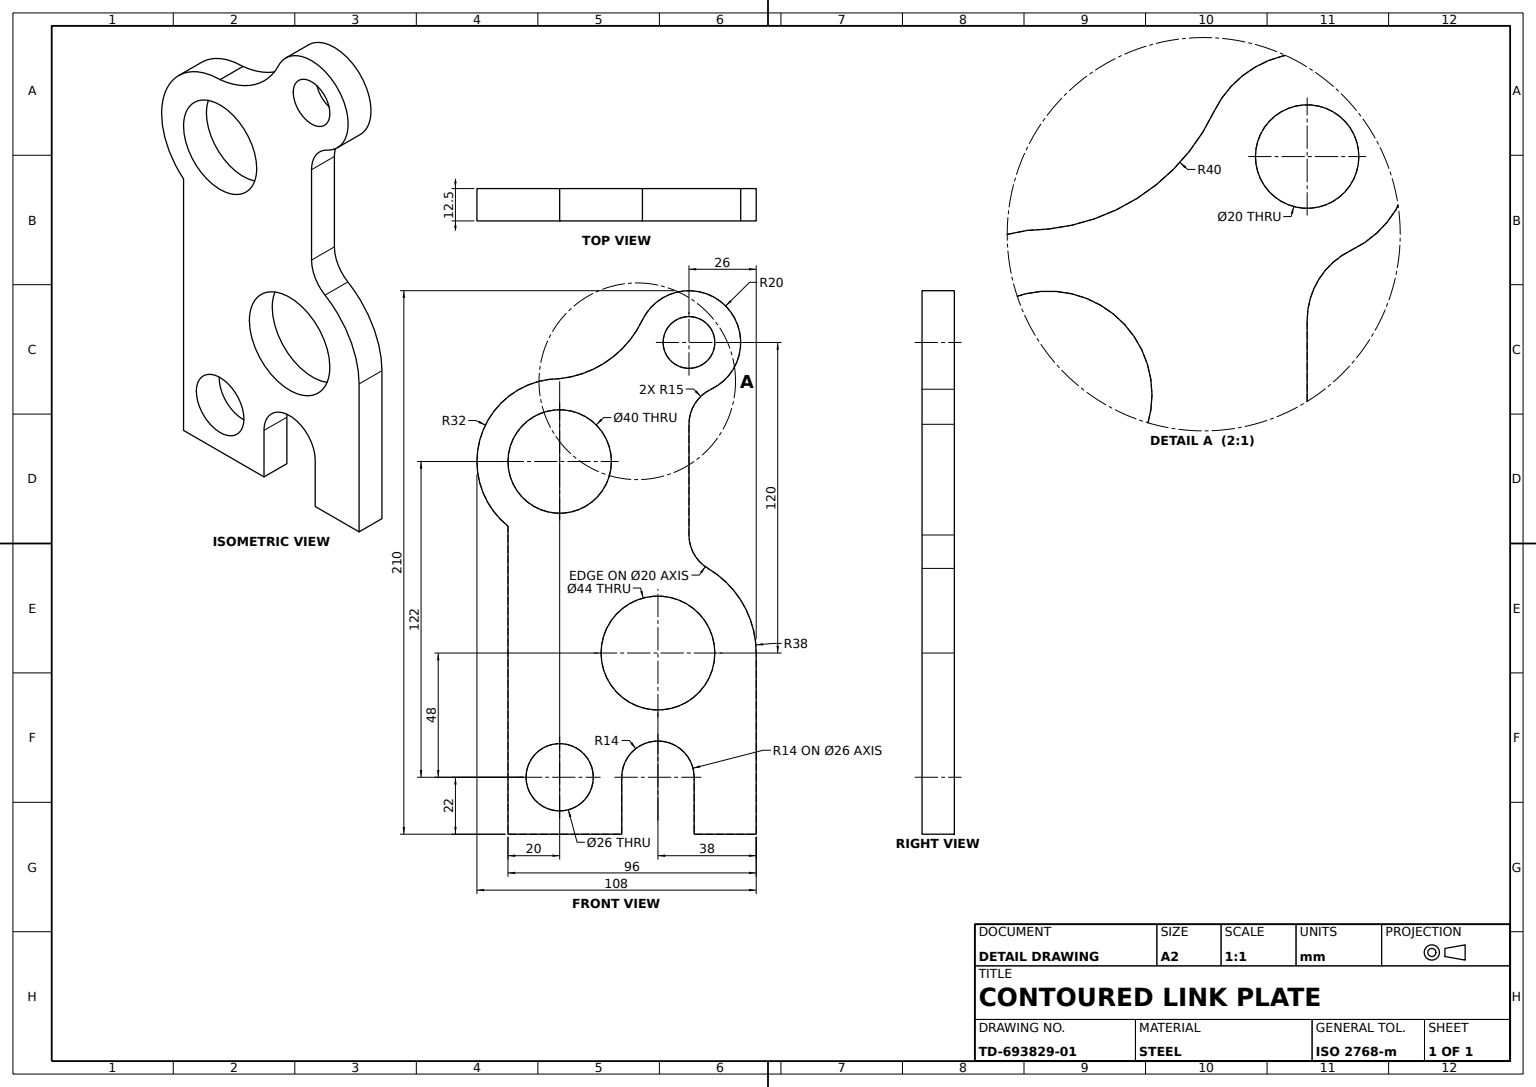
from build123d import *

# Parameters (mm, degrees)
BRACKET_PROFILE_SKETCH_R   = 13
BRACKET_PROFILE_SKETCH_R_2 = 20
BRACKET_PROFILE_SKETCH_R_3 = 10
BRACKET_PROFILE_SKETCH_R_4 = 22
BRACKET_PLATE_12_5MM_DEPTH = 12.5
EDGE_FILLET_R15_R          = 15


with BuildPart() as part:
    # Bracket Profile Sketch → Bracket Plate 12.5mm (new body)
    with BuildSketch(Plane.XY):
        with BuildLine():
            Line((0, 119.020008006), (0, 0))
            Line((0, 0), (44, 0))
            Line((44, 0), (44, 22))
            ThreePointArc((44, 22), (58, 36), (72, 22))
            Line((72, 22), (72, 0))
            Line((72, 0), (96, 0))
            Line((96, 0), (96, 70))
            ThreePointArc((96, 70), (91.01229045, 88.819901149), (77.358490566, 102.699370682))
            ThreePointArc((77.358490566, 102.699370682), (71.968832717, 108.178108656), (70, 115.607017004))
            Line((70, 115.607017004), (70, 170))
            ThreePointArc((70, 170), (86.946326412, 200.621771092), (52, 198.717797887))
            ThreePointArc((52, 198.717797887), (38.977494473, 183.164838251), (20, 176))
            ThreePointArc((20, 176), (-10.194037026, 154.598119083), (0, 119.020008006))
        make_face()
        with Locations((20, 22)):
            Circle(BRACKET_PROFILE_SKETCH_R, mode=Mode.SUBTRACT)
        with Locations((20, 144)):
            Circle(BRACKET_PROFILE_SKETCH_R_2, mode=Mode.SUBTRACT)
        with Locations((70, 190)):
            Circle(BRACKET_PROFILE_SKETCH_R_3, mode=Mode.SUBTRACT)
        with Locations((58, 70)):
            Circle(BRACKET_PROFILE_SKETCH_R_4, mode=Mode.SUBTRACT)
    extrude(amount=BRACKET_PLATE_12_5MM_DEPTH)

    # Edge Fillet R15
    edge_fillet_r15_edges = [part.edges().sort_by_distance(p)[0] for p in [
        (70, 170, 6.25),
    ]]
    fillet(edge_fillet_r15_edges, radius=EDGE_FILLET_R15_R)


solid = part.part
